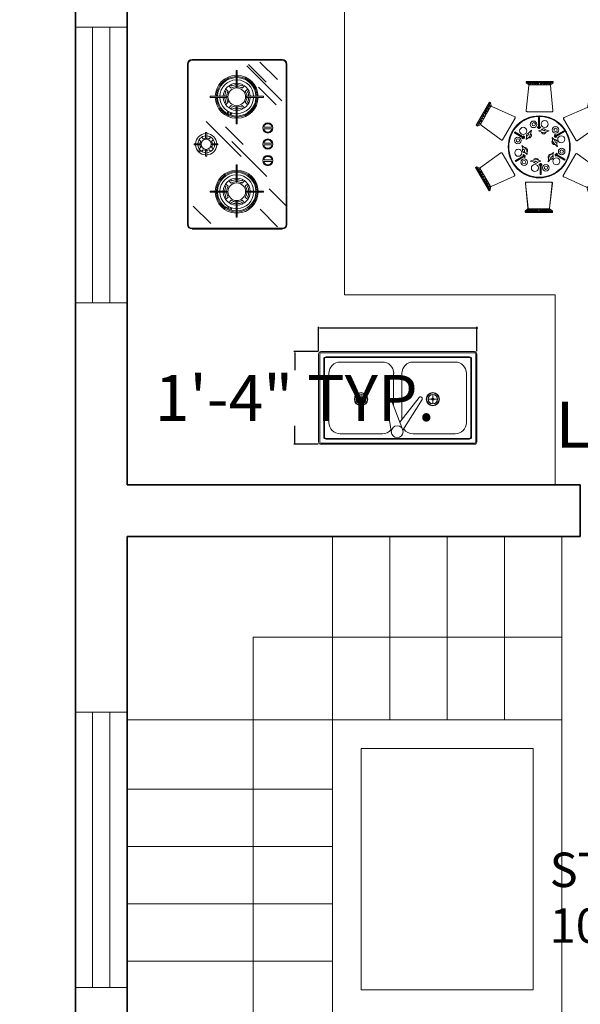
# Model space of a CAD drawing. Units: inches. Extents: x 125 to 976, y 231 to 853.
# Tile 13 of 16: x 557 to 655, y 413 to 584. Entities that reach past the tile are written whole.
import ezdxf

# ---------------------------------------------------------------- set-up
doc = ezdxf.new("R2010")
doc.units = ezdxf.units.IN
doc.header["$MEASUREMENT"] = 0
for name, color, linetype, lineweight in [('A-ANNO-DIMS', 2, 'Continuous', 18), ('A-AREA-IDEN', 7, 'Continuous', 18), ('A-EQPM', 8, 'Continuous', 15), ('A-FLOR-CASE', 32, 'Continuous', 18), ('A-FLOR-FIXT', 9, 'Continuous', 18), ('A-FLOR-STRS', 7, 'Continuous', 18), ('A-GLAZ', 4, 'Continuous', 18), ('A-WALL', 7, 'Continuous', 35), ('Furniture', 8, 'Continuous', 15)]:
    doc.layers.add(name, color=color, linetype=linetype, lineweight=lineweight)
doc.styles.get("Standard").update_dxf_attribs({"font": 'italic8.shx'})
doc.dimstyles.get("Standard").update_dxf_attribs({"dimtxt": 8, "dimasz": 0.18, "dimexe": 0.18, "dimexo": 0.0625, "dimgap": 0.09, "dimtad": 0, "dimtih": 1, "dimtoh": 1, "dimdec": 4, "dimzin": 0, "dimdsep": 46, "dimlunit": 3, "dimtxsty": 'Standard', "dimcen": 0.09, "dimclrt": 4, "dimadec": 0, "dimazin": 0, "dimtfac": 1, "dimtdec": 4, "dimtofl": 0, "dimtmove": 0, "dimatfit": 3, "dimfxl": 1, "dimtolj": 1, "dimtzin": 0, "dimarcsym": 0})

# ---------------------------------------------------------------- blocks, each defined once
blk = doc.blocks.new('DINING-SET-ROUND-6')
for p, q in [((8.8, 22.58), (9.2, 22.26)), ((8.83, 22.8), (8.83, 22.6)), ((13.52, 22.8), (8.83, 22.8)), ((8.83, 22.6), (13.52, 22.6)), ((9.19, 22.53), (9.57, 22.55)), ((9.54, 22.27), (9.19, 22.53)), ((9.57, 22.55), (9.56, 22.32)), ((9.67, 22.56), (9.91, 22.32)), ((9.8, 22.55), (9.89, 22.55)), ((10.04, 22.32), (9.8, 22.55)), ((9.89, 22.55), (10.01, 22.45)), ((9.91, 22.32), (10.04, 22.32)), ((10.01, 22.45), (10.04, 22.48)), ((10.04, 22.48), (10.05, 22.34)), ((10.15, 22.56), (10.39, 22.32)), ((10.28, 22.55), (10.37, 22.55)), ((10.52, 22.32), (10.28, 22.55)), ((10.37, 22.55), (10.49, 22.45)), ((10.39, 22.32), (10.52, 22.32)), ((10.49, 22.45), (10.52, 22.48)), ((10.52, 22.48), (10.54, 22.34)), ((10.63, 22.56), (10.87, 22.32)), ((10.76, 22.55), (10.86, 22.55)), ((11, 22.32), (10.76, 22.55)), ((10.86, 22.55), (10.97, 22.45)), ((10.87, 22.32), (11, 22.32)), ((10.97, 22.45), (11, 22.48)), ((11, 22.48), (11.02, 22.34)), ((11.32, 22.48), (11.31, 22.34)), ((11.32, 22.32), (11.56, 22.55)), ((11.35, 22.45), (11.32, 22.48)), ((11.45, 22.32), (11.32, 22.32)), ((11.47, 22.55), (11.35, 22.45)), ((11.69, 22.56), (11.45, 22.32)), ((11.56, 22.55), (11.47, 22.55)), ((11.8, 22.48), (11.79, 22.34)), ((11.8, 22.32), (12.04, 22.55)), ((11.83, 22.45), (11.8, 22.48)), ((11.93, 22.32), (11.8, 22.32)), ((11.95, 22.55), (11.83, 22.45)), ((12.17, 22.56), (11.93, 22.32)), ((12.04, 22.55), (11.95, 22.55)), ((12.28, 22.48), (12.27, 22.34)), ((12.28, 22.32), (12.52, 22.55)), ((12.32, 22.45), (12.28, 22.48)), ((12.41, 22.32), (12.28, 22.32)), ((12.43, 22.55), (12.32, 22.45)), ((12.65, 22.56), (12.41, 22.32)), ((12.52, 22.55), (12.43, 22.55)), ((12.75, 22.55), (12.77, 22.32)), ((13.13, 22.53), (12.75, 22.55)), ((12.78, 22.27), (13.13, 22.53)), ((13.52, 22.58), (13.12, 22.26)), ((13.52, 22.6), (13.52, 22.8)), ((8.82, 17.72), (9.3, 22.08)), ((9.2, 22.26), (9.54, 22.27)), ((9.46, 22.23), (12.91, 22.23)), ((13.12, 22.26), (12.78, 22.27)), ((13.07, 22.08), (13.49, 17.72)), ((2.44, 19.22), (0.09, 15.16)), ((0.27, 15.05), (2.62, 19.11)), ((2.62, 19.11), (2.44, 19.22)), ((2.63, 19.1), (2.71, 18.6)), ((19.62, 18.97), (19.54, 18.47)), ((19.83, 19.06), (19.65, 18.95)), ((19.65, 18.95), (21.99, 14.9)), ((22.17, 15), (19.83, 19.06)), ((0.91, 15.41), (2.63, 18.4)), ((1.66, 17.16), (1.62, 17.15)), ((1.68, 17.39), (1.63, 17.31)), ((1.63, 17.31), (1.66, 17.16)), ((1.75, 17.07), (1.68, 17.39)), ((1.73, 17.51), (1.82, 17.18)), ((1.82, 17.18), (1.75, 17.07)), ((1.9, 17.58), (1.86, 17.57)), ((1.86, 17.57), (1.97, 17.48)), ((1.92, 17.81), (1.87, 17.73)), ((1.87, 17.73), (1.9, 17.58)), ((1.99, 17.49), (1.92, 17.81)), ((1.97, 17.93), (2.06, 17.6)), ((2.06, 17.6), (1.99, 17.49)), ((2.14, 18), (2.1, 17.99)), ((2.1, 17.99), (2.21, 17.9)), ((2.16, 18.23), (2.11, 18.14)), ((2.11, 18.14), (2.14, 18)), ((2.24, 17.91), (2.16, 18.23)), ((2.21, 18.35), (2.3, 18.02)), ((2.3, 18.02), (2.24, 17.91)), ((2.48, 18.75), (2.27, 18.42)), ((2.27, 18.42), (2.48, 18.32)), ((2.53, 18.31), (2.48, 18.75)), ((2.71, 18.6), (2.53, 18.31)), ((2.84, 18.46), (6.82, 16.65)), ((13.33, 17.54), (8.98, 17.54)), ((15.42, 16.53), (19.43, 18.29)), ((19.54, 18.47), (19.72, 18.18)), ((19.64, 18.23), (21.36, 15.24)), ((19.72, 18.18), (19.77, 18.62)), ((19.77, 18.62), (19.97, 18.29)), ((19.97, 18.29), (19.77, 18.19)), ((20.03, 18.21), (19.95, 17.89)), ((19.95, 17.89), (20.01, 17.77)), ((20.01, 17.77), (20.08, 18.1)), ((20.15, 17.86), (20.03, 17.77)), ((20.08, 18.1), (20.13, 18.01)), ((20.13, 18.01), (20.11, 17.87)), ((20.11, 17.87), (20.15, 17.86)), ((20.28, 17.8), (20.19, 17.47)), ((20.19, 17.47), (20.25, 17.36)), ((20.25, 17.36), (20.33, 17.68)), ((20.39, 17.44), (20.27, 17.35)), ((20.33, 17.68), (20.37, 17.6)), ((20.37, 17.6), (20.35, 17.45)), ((20.35, 17.45), (20.39, 17.44)), ((20.52, 17.38), (20.43, 17.05)), ((20.49, 16.94), (20.57, 17.26)), ((20.57, 17.26), (20.61, 17.18)), ((20.61, 17.18), (20.59, 17.03)), ((0.51, 15.33), (0.69, 15.67)), ((0.91, 15.51), (0.51, 15.33)), ((0.69, 15.67), (0.87, 15.54)), ((0.72, 15.76), (1.05, 15.85)), ((0.75, 15.21), (0.91, 15.51)), ((1.11, 15.96), (0.8, 15.86)), ((0.8, 15.86), (0.85, 15.95)), ((0.85, 15.95), (0.99, 16)), ((0.96, 16.18), (1.29, 16.27)), ((0.97, 16.04), (1.11, 15.98)), ((0.99, 16), (0.97, 16.04)), ((1.35, 16.38), (1.04, 16.28)), ((1.04, 16.28), (1.09, 16.36)), ((1.05, 15.85), (1.11, 15.96)), ((1.09, 16.36), (1.23, 16.41)), ((1.2, 16.59), (1.53, 16.68)), ((1.23, 16.41), (1.21, 16.46)), ((1.21, 16.46), (1.35, 16.4)), ((1.59, 16.79), (1.28, 16.7)), ((1.28, 16.7), (1.33, 16.78)), ((1.29, 16.27), (1.35, 16.38)), ((1.33, 16.78), (1.47, 16.83)), ((1.45, 16.87), (1.59, 16.82)), ((1.47, 16.83), (1.45, 16.87)), ((1.53, 16.68), (1.59, 16.79)), ((1.62, 17.15), (1.73, 17.07)), ((6.9, 16.42), (4.72, 12.66)), ((10.97, 16.52, 0.91), (10.97, 14.61, 0.91)), ((11.03, 16.52, 0.91), (10.97, 16.52, 0.91)), ((11.03, 14.61, 0.91), (11.03, 16.52, 0.91)), ((11.08, 16.52, 0.91), (11.08, 14.61, 0.91)), ((11.14, 16.52, 0.91), (11.08, 16.52, 0.91)), ((11.14, 14.61, 0.91), (11.14, 16.52, 0.91)), ((17.52, 12.54), (15.34, 16.3)), ((20.43, 17.05), (20.49, 16.94)), ((20.63, 17.02), (20.51, 16.94)), ((20.59, 17.03), (20.63, 17.02)), ((20.65, 16.66), (20.97, 16.57)), ((20.72, 16.55), (20.65, 16.66)), ((20.79, 16.74), (20.66, 16.69)), ((21.05, 16.46), (20.72, 16.55)), ((20.78, 16.7), (20.79, 16.74)), ((20.92, 16.65), (20.78, 16.7)), ((20.89, 16.25), (21.21, 16.15)), ((20.96, 16.14), (20.89, 16.25)), ((21.03, 16.33), (20.9, 16.27)), ((20.97, 16.57), (20.92, 16.65)), ((21.29, 16.05), (20.96, 16.14)), ((21.02, 16.28), (21.03, 16.33)), ((21.16, 16.23), (21.02, 16.28)), ((21.13, 15.83), (21.45, 15.73)), ((21.2, 15.72), (21.13, 15.83)), ((21.27, 15.91), (21.14, 15.85)), ((21.21, 16.15), (21.16, 16.23)), ((21.53, 15.63), (21.2, 15.72)), ((21.26, 15.87), (21.27, 15.91)), ((21.4, 15.82), (21.26, 15.87)), ((21.56, 15.54), (21.37, 15.41)), ((21.45, 15.73), (21.4, 15.82)), ((21.74, 15.2), (21.56, 15.54)), ((0.09, 15.16), (0.27, 15.05)), ((0.27, 15.02), (0.75, 15.21)), ((4.49, 12.61), (0.95, 15.2)), ((6.8, 13.9, 0.91), (6.77, 13.85, 0.91)), ((6.77, 13.85, 0.91), (8.43, 12.89, 0.91)), ((8.46, 12.94, 0.91), (6.8, 13.9, 0.91)), ((6.86, 14, 0.91), (6.83, 13.95, 0.91)), ((6.83, 13.95, 0.91), (8.49, 12.99, 0.91)), ((8.52, 13.04, 0.91), (6.86, 14, 0.91)), ((9.74, 14.31, 0.91), (9.23, 13.78, 0.91)), ((9.23, 13.78, 0.91), (9.27, 13.54, 0.91)), ((9.58, 13.56, 0.91), (9.74, 14.31, 0.91)), ((10.81, 14.88, 0.91), (10.81, 14.72, 0.91)), ((10.97, 14.88, 0.91), (10.81, 14.88, 0.91)), ((10.81, 14.72, 0.91), (10.97, 14.72, 0.91)), ((10.97, 14.61, 0.91), (11.03, 14.61, 0.91)), ((11.61, 14.37, 0.91), (10.99, 14.19, 0.91)), ((10.99, 14.19, 0.91), (11.68, 13.89, 0.91)), ((11.08, 14.88, 0.91), (11.03, 14.88, 0.91)), ((11.03, 14.72, 0.91), (11.08, 14.72, 0.91)), ((11.08, 14.61, 0.91), (11.14, 14.61, 0.91)), ((11.31, 14.88, 0.91), (11.14, 14.88, 0.91)), ((11.14, 14.72, 0.91), (11.31, 14.72, 0.91)), ((11.31, 14.72, 0.91), (11.31, 14.88, 0.91)), ((11.94, 14.21, 0.91), (11.61, 14.37, 0.91)), ((11.68, 13.89, 0.91), (12.12, 13.95, 0.91)), ((12.14, 14.36, 0.91), (11.94, 14.21, 0.91)), ((12.12, 13.95, 0.91), (12.85, 14.19, 0.91)), ((12.85, 14.19, 0.91), (12.14, 14.36, 0.91)), ((15.38, 14.23, 0.91), (13.72, 13.27, 0.91)), ((13.75, 13.22, 0.91), (15.41, 14.18, 0.91)), ((15.44, 14.13, 0.91), (13.78, 13.17, 0.91)), ((13.81, 13.12, 0.91), (15.47, 14.08, 0.91)), ((15.41, 14.18, 0.91), (15.38, 14.23, 0.91)), ((15.47, 14.08, 0.91), (15.44, 14.13, 0.91)), ((21.32, 15.03), (17.75, 12.49)), ((21.34, 15.37), (21.74, 15.2)), ((21.5, 15.07), (21.34, 15.37)), ((21.97, 14.89), (21.5, 15.07)), ((21.99, 14.9), (22.17, 15)), ((8.2, 13.02, 0.91), (8.12, 12.89, 0.91)), ((8.12, 12.89, 0.91), (8.26, 12.81, 0.91)), ((8.26, 13.12, 0.91), (8.23, 13.07, 0.91)), ((8.26, 12.81, 0.91), (8.34, 12.95, 0.91)), ((8.37, 13.32, 0.91), (8.29, 13.17, 0.91)), ((8.51, 13.24, 0.91), (8.37, 13.32, 0.91)), ((8.37, 13, 0.91), (8.39, 13.04, 0.91)), ((8.42, 13.1, 0.91), (8.51, 13.24, 0.91)), ((8.43, 12.89, 0.91), (8.46, 12.94, 0.91)), ((8.49, 12.99, 0.91), (8.52, 13.04, 0.91)), ((8.96, 13.32, 0.91), (8.81, 12.7, 0.91)), ((8.81, 12.7, 0.91), (9.41, 13.15, 0.91)), ((9.27, 13.54, 0.91), (8.96, 13.32, 0.91)), ((9.41, 13.15, 0.91), (9.58, 13.56, 0.91)), ((13.84, 12.59, 0.91), (13.37, 13.04, 0.91)), ((13.37, 13.04, 0.91), (13.46, 12.29, 0.91)), ((13.46, 12.29, 0.91), (13.73, 11.94, 0.91)), ((13.72, 13.27, 0.91), (13.75, 13.22, 0.91)), ((13.88, 13.54, 0.91), (13.74, 13.46, 0.91)), ((13.74, 13.46, 0.91), (13.82, 13.33, 0.91)), ((13.78, 13.17, 0.91), (13.81, 13.12, 0.91)), ((13.87, 12.23, 0.91), (13.84, 12.59, 0.91)), ((13.85, 13.27, 0.91), (13.88, 13.23, 0.91)), ((14.09, 12.13, 0.91), (13.87, 12.23, 0.91)), ((13.96, 13.4, 0.91), (13.88, 13.54, 0.91)), ((13.91, 13.18, 0.91), (13.99, 13.03, 0.91)), ((14.01, 13.31, 0.91), (13.99, 13.35, 0.91)), ((13.99, 13.03, 0.91), (14.13, 13.11, 0.91)), ((14.13, 13.11, 0.91), (14.04, 13.25, 0.91)), ((14.3, 11.43, 0.91), (14.09, 12.13, 0.91)), ((0.85, 7.79), (4.42, 10.34)), ((8.08, 11.67, 0.91), (8.28, 10.97, 0.91)), ((8.64, 11.17, 0.91), (8.08, 11.67, 0.91)), ((8.28, 10.97, 0.91), (8.51, 10.88, 0.91)), ((8.51, 10.88, 0.91), (8.54, 10.51, 0.91)), ((8.54, 10.51, 0.91), (9, 10.06, 0.91)), ((8.92, 10.81, 0.91), (8.64, 11.17, 0.91)), ((9, 10.06, 0.91), (8.92, 10.81, 0.91)), ((13.57, 10.41, 0.91), (12.96, 9.95, 0.91)), ((13.41, 9.78, 0.91), (13.57, 10.41, 0.91)), ((13.73, 11.94, 0.91), (14.3, 11.43, 0.91)), ((14.12, 10.3, 0.91), (14.04, 10.16, 0.91)), ((14.25, 10.22, 0.91), (14.12, 10.3, 0.91)), ((4.65, 10.29), (6.83, 6.52)), ((8.57, 9.99, 0.91), (6.91, 9.03, 0.91)), ((6.91, 9.03, 0.91), (6.94, 8.97, 0.91)), ((6.94, 8.97, 0.91), (8.6, 9.93, 0.91)), ((8.62, 9.89, 0.91), (6.96, 8.93, 0.91)), ((6.96, 8.93, 0.91), (6.99, 8.88, 0.91)), ((6.99, 8.88, 0.91), (8.65, 9.84, 0.91)), ((8.38, 10.07, 0.91), (8.25, 10, 0.91)), ((8.25, 10, 0.91), (8.33, 9.85, 0.91)), ((8.36, 9.8, 0.91), (8.39, 9.75, 0.91)), ((8.47, 9.93, 0.91), (8.38, 10.07, 0.91)), ((8.42, 9.7, 0.91), (8.5, 9.57, 0.91)), ((8.53, 9.83, 0.91), (8.5, 9.88, 0.91)), ((8.5, 9.57, 0.91), (8.63, 9.64, 0.91)), ((8.63, 9.64, 0.91), (8.56, 9.78, 0.91)), ((8.6, 9.93, 0.91), (8.57, 9.99, 0.91)), ((8.65, 9.84, 0.91), (8.62, 9.89, 0.91)), ((10.25, 9.16, 0.91), (9.53, 8.92, 0.91)), ((9.53, 8.92, 0.91), (10.24, 8.75, 0.91)), ((10.24, 8.75, 0.91), (10.43, 8.9, 0.91)), ((10.69, 9.22, 0.91), (10.25, 9.16, 0.91)), ((10.43, 8.9, 0.91), (10.77, 8.74, 0.91)), ((11.39, 8.92, 0.91), (10.69, 9.22, 0.91)), ((10.77, 8.74, 0.91), (11.39, 8.92, 0.91)), ((12.79, 9.54, 0.91), (12.64, 8.8, 0.91)), ((12.64, 8.8, 0.91), (13.14, 9.33, 0.91)), ((12.96, 9.95, 0.91), (12.79, 9.54, 0.91)), ((13.11, 9.57, 0.91), (13.41, 9.78, 0.91)), ((13.14, 9.33, 0.91), (13.11, 9.57, 0.91)), ((13.88, 10.12, 0.91), (13.85, 10.07, 0.91)), ((13.85, 10.07, 0.91), (15.52, 9.11, 0.91)), ((13.95, 10.01, 0.91), (13.87, 9.86, 0.91)), ((13.87, 9.86, 0.91), (14, 9.79, 0.91)), ((15.55, 9.16, 0.91), (13.88, 10.12, 0.91)), ((13.94, 10.22, 0.91), (13.91, 10.17, 0.91)), ((13.91, 10.17, 0.91), (15.57, 9.21, 0.91)), ((15.6, 9.26, 0.91), (13.94, 10.22, 0.91)), ((14.01, 10.11, 0.91), (13.98, 10.06, 0.91)), ((14, 9.79, 0.91), (14.09, 9.93, 0.91)), ((14.12, 9.98, 0.91), (14.15, 10.03, 0.91)), ((14.18, 10.08, 0.91), (14.25, 10.22, 0.91)), ((15.28, 6.4), (17.45, 10.17)), ((15.52, 9.11, 0.91), (15.55, 9.16, 0.91)), ((15.57, 9.21, 0.91), (15.6, 9.26, 0.91)), ((17.68, 10.22), (21.22, 7.62)), ((0.18, 7.93), (0, 7.82)), ((0, 7.82), (2.35, 3.77)), ((2.53, 3.87), (0.18, 7.93)), ((0.2, 7.94), (0.68, 7.75)), ((0.43, 7.63), (0.61, 7.29)), ((0.83, 7.45), (0.43, 7.63)), ((0.61, 7.29), (0.8, 7.41)), ((0.64, 7.19), (0.97, 7.11)), ((0.68, 7.75), (0.83, 7.45)), ((0.72, 7.09), (0.77, 7.01)), ((1.04, 6.99), (0.72, 7.09)), ((0.77, 7.01), (0.91, 6.96)), ((2.53, 4.6), (0.81, 7.58)), ((0.9, 6.91), (1.03, 6.97)), ((0.91, 6.96), (0.9, 6.91)), ((0.97, 7.11), (1.04, 6.99)), ((11.23, 8.39, 0.91), (11.07, 8.39, 0.91)), ((11.07, 8.39, 0.91), (11.07, 8.23, 0.91)), ((11.07, 8.23, 0.91), (11.23, 8.23, 0.91)), ((11.29, 8.5, 0.91), (11.23, 8.5, 0.91)), ((11.23, 8.5, 0.91), (11.23, 6.58, 0.91)), ((11.29, 6.58, 0.91), (11.29, 8.5, 0.91)), ((11.35, 8.39, 0.91), (11.29, 8.39, 0.91)), ((11.29, 8.23, 0.91), (11.35, 8.23, 0.91)), ((11.41, 8.5, 0.91), (11.35, 8.5, 0.91)), ((11.35, 8.5, 0.91), (11.35, 6.58, 0.91)), ((11.41, 6.58, 0.91), (11.41, 8.5, 0.91)), ((11.56, 8.39, 0.91), (11.41, 8.39, 0.91)), ((11.41, 8.23, 0.91), (11.56, 8.23, 0.91)), ((11.56, 8.23, 0.91), (11.56, 8.39, 0.91)), ((21.26, 7.41), (19.54, 4.43)), ((21.9, 7.77), (19.55, 3.71)), ((19.73, 3.61), (22.08, 7.67)), ((21.12, 6.98), (21.06, 6.86)), ((21.06, 6.86), (21.37, 6.96)), ((21.45, 7.06), (21.12, 6.98)), ((21.33, 6.88), (21.19, 6.83)), ((21.42, 7.62), (21.27, 7.32)), ((21.27, 7.32), (21.66, 7.5)), ((21.49, 7.15), (21.3, 7.28)), ((21.37, 6.96), (21.33, 6.88)), ((21.9, 7.81), (21.42, 7.62)), ((21.66, 7.5), (21.49, 7.15)), ((22.08, 7.67), (21.9, 7.77)), ((0.88, 6.78), (1.21, 6.69)), ((0.96, 6.67), (1.01, 6.59)), ((1.28, 6.58), (0.96, 6.67)), ((1.01, 6.59), (1.15, 6.54)), ((1.13, 6.36), (1.45, 6.27)), ((1.14, 6.5), (1.27, 6.56)), ((1.15, 6.54), (1.14, 6.5)), ((1.2, 6.26), (1.25, 6.17)), ((1.52, 6.16), (1.2, 6.26)), ((1.21, 6.69), (1.28, 6.58)), ((1.25, 6.17), (1.39, 6.12)), ((1.38, 6.08), (1.51, 6.14)), ((1.39, 6.12), (1.38, 6.08)), ((1.45, 6.27), (1.52, 6.16)), ((1.54, 5.8), (1.66, 5.89)), ((1.58, 5.79), (1.54, 5.8)), ((1.56, 5.65), (1.58, 5.79)), ((1.6, 5.56), (1.56, 5.65)), ((1.68, 5.88), (1.6, 5.56)), ((1.65, 5.44), (1.74, 5.77)), ((1.74, 5.77), (1.68, 5.88)), ((1.78, 5.39), (1.9, 5.47)), ((1.82, 5.37), (1.78, 5.39)), ((1.8, 5.23), (1.82, 5.37)), ((1.85, 5.15), (1.8, 5.23)), ((1.92, 5.47), (1.85, 5.15)), ((1.9, 5.03), (1.98, 5.35)), ((1.98, 5.35), (1.92, 5.47)), ((6.75, 6.3), (2.74, 4.53)), ((8.84, 5.28), (13.19, 5.28)), ((8.89, 5.26), (13.23, 5.26)), ((11.23, 6.58, 0.91), (11.29, 6.58, 0.91)), ((11.35, 6.58, 0.91), (11.41, 6.58, 0.91)), ((19.33, 4.36), (15.35, 6.18)), ((20.11, 5.22), (20.18, 5.34)), ((20.2, 4.9), (20.11, 5.22)), ((20.18, 5.34), (20.25, 5.01)), ((20.31, 5.26), (20.2, 5.34)), ((20.27, 5.24), (20.31, 5.26)), ((20.3, 5.1), (20.27, 5.24)), ((20.35, 5.64), (20.42, 5.75)), ((20.44, 5.31), (20.35, 5.64)), ((20.42, 5.75), (20.49, 5.43)), ((20.56, 5.67), (20.44, 5.76)), ((20.49, 5.43), (20.54, 5.51)), ((20.51, 5.66), (20.56, 5.67)), ((20.54, 5.51), (20.51, 5.66)), ((20.64, 6.14), (20.58, 6.03)), ((20.58, 6.03), (20.89, 6.13)), ((20.72, 5.95), (20.58, 6.01)), ((20.97, 6.23), (20.64, 6.14)), ((20.84, 6.04), (20.7, 5.99)), ((20.7, 5.99), (20.72, 5.95)), ((20.88, 6.56), (20.82, 6.45)), ((20.82, 6.45), (21.13, 6.54)), ((20.96, 6.37), (20.82, 6.43)), ((20.89, 6.13), (20.84, 6.04)), ((21.21, 6.65), (20.88, 6.56)), ((21.08, 6.46), (20.94, 6.41)), ((20.94, 6.41), (20.96, 6.37)), ((21.2, 6.78), (21.06, 6.84)), ((21.13, 6.54), (21.08, 6.46)), ((21.19, 6.83), (21.2, 6.78)), ((2.02, 4.97), (2.14, 5.06)), ((2.07, 4.96), (2.02, 4.97)), ((2.04, 4.81), (2.07, 4.96)), ((2.09, 4.73), (2.04, 4.81)), ((2.16, 5.05), (2.09, 4.73)), ((2.14, 4.61), (2.22, 4.94)), ((2.22, 4.94), (2.16, 5.05)), ((2.2, 4.53), (2.4, 4.63)), ((2.4, 4.21), (2.2, 4.53)), ((2.35, 3.77), (2.53, 3.87)), ((2.45, 4.64), (2.4, 4.21)), ((2.63, 4.36), (2.45, 4.64)), ((2.56, 3.85), (2.63, 4.36)), ((9.1, 0.74), (8.68, 5.1)), ((9.14, 0.73), (8.73, 5.09)), ((13.35, 5.1), (12.87, 0.74)), ((13.39, 5.09), (12.91, 0.72)), ((19.46, 4.23), (19.64, 4.51)), ((19.54, 3.72), (19.46, 4.23)), ((19.55, 3.71), (19.73, 3.61)), ((19.64, 4.51), (19.69, 4.08)), ((19.9, 4.4), (19.69, 4.5)), ((19.69, 4.08), (19.9, 4.4)), ((19.87, 4.81), (19.94, 4.92)), ((19.96, 4.48), (19.87, 4.81)), ((19.94, 4.92), (20.01, 4.6)), ((20.07, 4.84), (19.96, 4.92)), ((20.01, 4.6), (20.06, 4.68)), ((20.03, 4.83), (20.07, 4.84)), ((20.06, 4.68), (20.03, 4.83)), ((20.25, 5.01), (20.3, 5.1)), ((8.65, 0.24), (9.05, 0.57)), ((8.65, 0.23), (8.65, 0.02)), ((13.34, 0.23), (8.65, 0.23)), ((8.65, 0.02), (13.34, 0.02)), ((8.69, 0.23), (9.09, 0.55)), ((8.69, 0.21), (8.69, 0)), ((13.38, 0.21), (8.69, 0.21)), ((8.69, 0), (13.38, 0)), ((9.39, 0.55), (9.04, 0.29)), ((9.04, 0.29), (9.42, 0.28)), ((9.05, 0.57), (9.39, 0.55)), ((9.43, 0.53), (9.08, 0.28)), ((9.08, 0.28), (9.46, 0.26)), ((9.09, 0.55), (9.43, 0.53)), ((12.71, 0.6), (9.26, 0.6)), ((12.75, 0.58), (9.3, 0.58)), ((9.42, 0.28), (9.41, 0.5)), ((9.46, 0.26), (9.45, 0.49)), ((9.52, 0.26), (9.76, 0.5)), ((9.56, 0.25), (9.8, 0.49)), ((9.89, 0.5), (9.65, 0.28)), ((9.65, 0.28), (9.74, 0.28)), ((9.93, 0.49), (9.69, 0.26)), ((9.69, 0.26), (9.78, 0.26)), ((9.74, 0.28), (9.85, 0.37)), ((9.76, 0.5), (9.89, 0.5)), ((9.78, 0.26), (9.9, 0.36)), ((9.8, 0.49), (9.93, 0.49)), ((9.85, 0.37), (9.89, 0.34)), ((9.89, 0.34), (9.9, 0.49)), ((9.9, 0.36), (9.93, 0.33)), ((9.93, 0.33), (9.94, 0.47)), ((10, 0.26), (10.24, 0.5)), ((10.04, 0.25), (10.28, 0.49)), ((10.37, 0.5), (10.13, 0.28)), ((10.13, 0.28), (10.22, 0.28)), ((10.41, 0.49), (10.17, 0.26)), ((10.17, 0.26), (10.27, 0.26)), ((10.22, 0.28), (10.34, 0.37)), ((10.24, 0.5), (10.37, 0.5)), ((10.27, 0.26), (10.38, 0.36)), ((10.28, 0.49), (10.41, 0.49)), ((10.34, 0.37), (10.37, 0.34)), ((10.37, 0.34), (10.38, 0.49)), ((10.38, 0.36), (10.41, 0.33)), ((10.41, 0.33), (10.43, 0.47)), ((10.48, 0.26), (10.72, 0.5)), ((10.52, 0.25), (10.76, 0.49)), ((10.85, 0.5), (10.61, 0.28)), ((10.61, 0.28), (10.71, 0.28)), ((10.89, 0.49), (10.65, 0.26)), ((10.65, 0.26), (10.75, 0.26)), ((10.71, 0.28), (10.82, 0.37)), ((10.72, 0.5), (10.85, 0.5)), ((10.75, 0.26), (10.86, 0.36)), ((10.76, 0.49), (10.89, 0.49)), ((10.82, 0.37), (10.85, 0.34)), ((10.85, 0.34), (10.87, 0.49)), ((10.86, 0.36), (10.89, 0.33)), ((10.89, 0.33), (10.91, 0.47)), ((11.17, 0.34), (11.15, 0.49)), ((11.17, 0.5), (11.41, 0.28)), ((11.3, 0.5), (11.17, 0.5)), ((11.2, 0.37), (11.17, 0.34)), ((11.21, 0.33), (11.2, 0.47)), ((11.31, 0.28), (11.2, 0.37)), ((11.21, 0.49), (11.45, 0.26)), ((11.34, 0.49), (11.21, 0.49)), ((11.24, 0.36), (11.21, 0.33)), ((11.36, 0.26), (11.24, 0.36)), ((11.54, 0.26), (11.3, 0.5)), ((11.41, 0.28), (11.31, 0.28)), ((11.58, 0.25), (11.34, 0.49)), ((11.45, 0.26), (11.36, 0.26)), ((11.65, 0.34), (11.64, 0.49)), ((11.65, 0.5), (11.89, 0.28)), ((11.78, 0.5), (11.65, 0.5)), ((11.68, 0.37), (11.65, 0.34)), ((11.69, 0.33), (11.68, 0.47)), ((11.8, 0.28), (11.68, 0.37)), ((11.69, 0.49), (11.93, 0.26)), ((11.82, 0.49), (11.69, 0.49)), ((11.73, 0.36), (11.69, 0.33)), ((11.84, 0.26), (11.73, 0.36)), ((12.02, 0.26), (11.78, 0.5)), ((11.89, 0.28), (11.8, 0.28)), ((12.06, 0.25), (11.82, 0.49)), ((11.93, 0.26), (11.84, 0.26)), ((12.13, 0.34), (12.12, 0.49)), ((12.13, 0.5), (12.37, 0.28)), ((12.26, 0.5), (12.13, 0.5)), ((12.17, 0.37), (12.13, 0.34)), ((12.17, 0.33), (12.16, 0.47)), ((12.17, 0.49), (12.42, 0.26)), ((12.3, 0.49), (12.17, 0.49)), ((12.28, 0.28), (12.17, 0.37)), ((12.21, 0.36), (12.17, 0.33)), ((12.32, 0.26), (12.21, 0.36)), ((12.5, 0.26), (12.26, 0.5)), ((12.37, 0.28), (12.28, 0.28)), ((12.54, 0.25), (12.3, 0.49)), ((12.42, 0.26), (12.32, 0.26)), ((12.6, 0.28), (12.61, 0.5)), ((12.98, 0.29), (12.6, 0.28)), ((12.97, 0.57), (12.63, 0.55)), ((12.63, 0.55), (12.98, 0.29)), ((12.64, 0.26), (12.66, 0.49)), ((13.02, 0.28), (12.64, 0.26)), ((13.01, 0.55), (12.67, 0.53)), ((12.67, 0.53), (13.02, 0.28)), ((13.37, 0.24), (12.97, 0.57)), ((13.41, 0.23), (13.01, 0.55)), ((13.34, 0.02), (13.34, 0.23)), ((13.38, 0), (13.38, 0.21))]:
    blk.add_line(p, q)
for centre, radius in [((11.09, 11.41), 5.4), ((11.09, 11.41), 5.3), ((10.11, 15.33, 0.91), 0.572), ((10.13, 15.34, 0.91), 0.295), ((12.04, 15.38, 0.91), 0.616), ((8.3, 14.2, 0.91), 0.616), ((13.92, 14.37, 0.91), 0.572), ((13.94, 14.37, 0.91), 0.295), ((7.38, 12.51, 0.91), 0.572), ((7.38, 12.53, 0.91), 0.295), ((14.93, 12.73, 0.91), 0.616), ((7.45, 10.38, 0.91), 0.616), ((15, 10.59, 0.91), 0.572), ((15, 10.58, 0.91), 0.295), ((8.45, 8.73, 0.91), 0.572), ((8.44, 8.74, 0.91), 0.295), ((14.08, 8.9, 0.91), 0.616), ((10.34, 7.73, 0.91), 0.616), ((12.26, 7.77, 0.91), 0.572), ((12.25, 7.77, 0.91), 0.295)]:
    blk.add_circle(centre, radius)
for centre, radius, start, end in [((9.46, 22.07), 0.16, 90, 173.7428), ((12.91, 22.07), 0.16, 5.4801, 90), ((2.77, 18.32), 0.16, 65.4801, 150), ((8.98, 17.7), 0.16, 173.7428, 270), ((13.33, 17.7), 0.16, 270, 5.4801), ((19.5, 18.15), 0.16, 30, 113.7428), ((6.76, 16.5), 0.16, 330, 65.4801), ((15.48, 16.38), 0.16, 113.7428, 210), ((1.05, 15.33), 0.16, 150, 233.7428), ((9.3, 13.42, 0.91), 0.448, 86.6641, 214.1442), ((9.3, 13.42, 0.91), 0.448, 257.0611, 44.0662), ((11.86, 14.13, 0.91), 0.448, 197.0611, 344.0662), ((11.86, 14.13, 0.91), 0.448, 26.6641, 154.1442), ((21.22, 15.16), 0.16, 305.4801, 30), ((4.58, 12.74), 0.16, 233.7428, 330), ((13.76, 12.26, 0.91), 0.448, 137.0611, 284.0662), ((13.76, 12.26, 0.91), 0.448, 326.6641, 94.1442), ((17.66, 12.62), 0.16, 210, 305.4801), ((4.52, 10.21), 0.16, 30, 125.4801), ((8.62, 10.85, 0.91), 0.448, 146.6641, 274.1442), ((8.62, 10.85, 0.91), 0.448, 317.0611, 104.0662), ((10.51, 8.98, 0.91), 0.448, 17.0611, 164.0662), ((10.51, 8.98, 0.91), 0.448, 206.6641, 334.1442), ((13.08, 9.68, 0.91), 0.448, 77.0611, 224.0662), ((13.08, 9.68, 0.91), 0.448, 266.6641, 34.1442), ((17.59, 10.09), 0.16, 53.7428, 150), ((0.95, 7.66), 0.16, 125.4801, 210), ((21.13, 7.49), 0.16, 330, 53.7428), ((6.69, 6.44), 0.16, 293.7428, 30), ((8.84, 5.12), 0.16, 90, 185.4801), ((8.89, 5.1), 0.16, 90, 185.4801), ((13.19, 5.12), 0.16, 353.7428, 90), ((13.23, 5.1), 0.16, 353.7428, 90), ((15.41, 6.32), 0.16, 150, 245.4801), ((2.67, 4.68), 0.16, 210, 293.7428), ((19.4, 4.51), 0.16, 245.4801, 330), ((9.26, 0.76), 0.16, 185.4801, 270), ((9.3, 0.74), 0.16, 185.4801, 270), ((12.71, 0.76), 0.16, 270, 353.7428), ((12.75, 0.74), 0.16, 270, 353.7428)]:
    blk.add_arc(centre, radius, start, end)
blk = doc.blocks.new('SINK-DOUBLE')
for p, q in [((0, 15.74), (0, 0.39)), ((0.2, 15.74), (0.2, 0.39)), ((27.17, 16.14), (0.4, 16.14)), ((27.17, 15.94), (0.4, 15.94)), ((27.37, 0.39), (27.37, 15.74)), ((27.56, 0.39), (27.56, 15.74)), ((0.91, 14.84), (0.91, 1.3)), ((1.03, 14.84), (1.03, 1.3)), ((26.26, 15.23), (1.3, 15.23)), ((26.26, 15.11), (1.3, 15.11)), ((11.11, 14.33), (3.78, 14.33)), ((23.78, 14.33), (16.46, 14.33)), ((26.54, 1.3), (26.54, 14.84)), ((26.66, 1.3), (26.66, 14.84)), ((1.81, 12.36), (1.81, 3.78)), ((13.07, 6.7), (13.07, 12.36)), ((14.49, 12.36), (14.49, 4.26)), ((25.75, 3.78), (25.75, 12.36)), ((7.39, 8.06), (7.39, 8.65)), ((19.9, 8.06), (19.9, 8.65)), ((7.18, 7.86), (6.59, 7.86)), ((7.39, 7.65), (7.39, 7.06)), ((7.59, 7.86), (8.18, 7.86)), ((11.9, 7.12), (12.69, 1.93)), ((12.59, 7.48), (12.04, 7.34)), ((14.68, 2.43), (12.83, 7.36)), ((14.16, 3.83), (17.49, 8.16)), ((14.68, 2.43), (18.03, 7.78)), ((17.92, 8.22), (17.95, 8.2)), ((19.7, 7.86), (19.11, 7.86)), ((19.9, 7.65), (19.9, 7.06)), ((20.11, 7.86), (20.7, 7.86)), ((3.78, 1.81), (11.11, 1.81)), ((16.46, 1.81), (23.78, 1.81)), ((0.4, 0.19), (27.17, 0.19)), ((1.3, 1.02), (26.26, 1.02)), ((1.3, 0.9), (26.26, 0.9)), ((0.4, 0), (27.17, 0))]:
    blk.add_line(p, q)
for centre, radius in [((7.39, 7.86), 1.16), ((7.39, 7.86), 1.1), ((7.39, 7.86), 0.83), ((7.39, 7.86), 0.794), ((19.9, 7.86), 1.16), ((19.9, 7.86), 1.1), ((19.9, 7.86), 0.83), ((19.9, 7.86), 0.794), ((7.39, 7.86), 0.204), ((7.39, 7.86), 0.0958), ((19.9, 7.86), 0.204), ((19.9, 7.86), 0.0958), ((13.69, 2.18), 1.03)]:
    blk.add_circle(centre, radius)
for centre, radius, start, end in [((0.4, 15.74), 0.394, 90, 180), ((0.4, 15.74), 0.197, 90, 180), ((27.17, 15.74), 0.394, 0, 90), ((27.17, 15.74), 0.197, 0, 90), ((1.3, 14.84), 0.394, 90, 180), ((1.3, 14.84), 0.276, 90, 180), ((3.78, 12.36), 1.97, 90, 180), ((11.11, 12.36), 1.97, 0, 90), ((16.46, 12.36), 1.97, 90, 180), ((23.78, 12.36), 1.97, 0, 90), ((26.26, 14.84), 0.394, 0, 90), ((26.26, 14.84), 0.276, 0, 90), ((12.09, 7.15), 0.197, 104.3233, 188.6985), ((12.64, 7.29), 0.197, 20.6498, 104.3233), ((17.74, 7.97), 0.315, 53.6309, 142.4185), ((17.76, 7.95), 0.315, 327.9301, 53.6309), ((3.78, 3.78), 1.97, 180, 270), ((23.78, 3.78), 1.97, 270, 0), ((11.11, 3.78), 1.97, 270, 319.575), ((16.46, 3.78), 1.97, 214.0864, 270), ((0.4, 0.39), 0.394, 180, 270), ((0.4, 0.39), 0.197, 180, 270), ((1.3, 1.3), 0.394, 180, 270), ((1.3, 1.3), 0.276, 180, 270), ((26.26, 1.3), 0.276, 270, 0), ((26.26, 1.3), 0.394, 270, 0), ((27.17, 0.39), 0.197, 270, 0), ((27.17, 0.39), 0.394, 270, 0)]:
    blk.add_arc(centre, radius, start, end)
blk = doc.blocks.new('COOKTOP-3BURNER')
for p, q in [((16.54, 29.53), (0.79, 29.53)), ((16.54, 29.41), (0.79, 29.41)), ((0, 28.74), (0, 0.79)), ((0.12, 28.74), (0.12, 0.79)), ((8.48, 24.8), (8.48, 27.63)), ((8.48, 27.63), (8.68, 27.63)), ((8.68, 24.8), (8.68, 27.63)), ((16.45, 22.35), (10.36, 28.44)), ((13.7, 25.61), (10.65, 28.66)), ((15.67, 26.04), (12.63, 29.08)), ((17.21, 0.79), (17.21, 28.74)), ((17.33, 0.79), (17.33, 28.74)), ((6.48, 24.12), (6.69, 23.92)), ((6.65, 24.4), (7.08, 23.97)), ((7.21, 24.95), (7.63, 24.53)), ((7.49, 25.12), (7.69, 24.92)), ((9.67, 25.12), (9.46, 24.92)), ((9.95, 24.95), (9.52, 24.53)), ((10.5, 24.4), (10.08, 23.97)), ((10.67, 24.12), (10.47, 23.92)), ((15.44, 21.65), (12.39, 24.7)), ((6.81, 23.13), (3.94, 23.13)), ((3.94, 23.13), (3.94, 22.93)), ((6.81, 22.93), (3.94, 22.93)), ((10.35, 23.13), (13.24, 23.13)), ((10.35, 22.93), (13.24, 22.93)), ((13.24, 23.13), (13.24, 22.93)), ((6.69, 22.14), (6.48, 21.94)), ((7.08, 22.09), (6.65, 21.66)), ((7.63, 21.53), (7.21, 21.1)), ((7.69, 21.14), (7.49, 20.93)), ((8.48, 21.26), (8.48, 18.35)), ((8.68, 21.26), (8.68, 18.35)), ((9.46, 21.14), (9.67, 20.93)), ((9.52, 21.53), (9.95, 21.1)), ((10.08, 22.09), (10.5, 21.66)), ((10.47, 22.14), (10.67, 21.94)), ((9.35, 12.64), (3.25, 18.73)), ((9.7, 14.73), (6.65, 17.78)), ((8.48, 18.35), (8.68, 18.35)), ((13.4, 17.77), (14.61, 17.77)), ((13.4, 17.46), (14.61, 17.46)), ((2.31, 15.27), (2.02, 15.56)), ((2.75, 15.72), (2.47, 16)), ((3.16, 16.82), (3.36, 16.82)), ((3.16, 15.84), (3.16, 16.82)), ((3.36, 15.84), (3.36, 16.82)), ((4.05, 16), (3.76, 15.72)), ((4.5, 15.56), (4.21, 15.27)), ((1.16, 14.86), (1.16, 14.67)), ((2.18, 14.86), (1.16, 14.86)), ((2.18, 14.67), (1.16, 14.67)), ((2.31, 14.26), (2.02, 13.97)), ((2.75, 13.81), (2.47, 13.53)), ((4.05, 13.53), (3.76, 13.81)), ((4.5, 13.97), (4.21, 14.26)), ((4.34, 14.86), (5.29, 14.86)), ((4.34, 14.67), (5.29, 14.67)), ((5.29, 14.86), (5.29, 14.67)), ((13.81, 9.14), (7.72, 15.23)), ((13.4, 14.96), (14.61, 14.96)), ((13.4, 14.65), (14.61, 14.65)), ((3.16, 13.69), (3.16, 12.69)), ((3.36, 12.69), (3.16, 12.69)), ((3.36, 13.69), (3.36, 12.69)), ((13.4, 12.07), (14.61, 12.07)), ((8.48, 11.18), (8.68, 11.18)), ((8.48, 8.27), (8.48, 11.18)), ((8.68, 8.27), (8.68, 11.18)), ((13.4, 11.76), (14.61, 11.76)), ((7.69, 8.39), (7.49, 8.59)), ((9.46, 8.39), (9.67, 8.59)), ((6.69, 7.39), (6.48, 7.59)), ((7.08, 7.44), (6.65, 7.87)), ((7.63, 8), (7.21, 8.42)), ((9.52, 8), (9.95, 8.42)), ((10.08, 7.44), (10.5, 7.87)), ((10.47, 7.39), (10.67, 7.59)), ((17.27, 3.97), (14.22, 7.02)), ((6.81, 6.6), (3.94, 6.6)), ((3.94, 6.4), (3.94, 6.6)), ((6.81, 6.4), (3.94, 6.4)), ((6.48, 5.41), (6.69, 5.61)), ((6.65, 5.13), (7.08, 5.56)), ((10.5, 5.13), (10.08, 5.56)), ((10.35, 6.6), (13.24, 6.6)), ((10.35, 6.4), (13.24, 6.4)), ((10.67, 5.41), (10.47, 5.61)), ((13.24, 6.4), (13.24, 6.6)), ((4.07, 0.94), (1.02, 3.99)), ((7.21, 4.57), (7.63, 5)), ((7.49, 4.4), (7.69, 4.61)), ((8.48, 4.93), (8.48, 2.09)), ((8.68, 4.93), (8.68, 2.09)), ((9.67, 4.4), (9.46, 4.61)), ((9.95, 4.57), (9.52, 5)), ((15.71, 0.4), (12.67, 3.44)), ((8.48, 2.09), (8.68, 2.09)), ((0.79, 0.12), (16.54, 0.12)), ((0.79, 0), (16.54, 0))]:
    blk.add_line(p, q)
for centre, radius in [((8.58, 23.03), 1.54), ((7.06, 20.26), 0.147), ((7.58, 20.04), 0.147), ((14, 17.61), 0.886), ((14, 17.61), 0.846), ((3.26, 14.76), 0.881), ((14, 14.8), 0.886), ((14, 14.8), 0.846), ((2.12, 13.62), 0.147), ((14, 11.92), 0.886), ((14, 11.92), 0.846), ((8.58, 6.5), 1.54), ((7.03, 3.73), 0.147), ((7.55, 3.51), 0.147)]:
    blk.add_circle(centre, radius)
for centre, radius, start, end in [((0.79, 28.74), 0.787, 90, 180), ((0.79, 28.74), 0.669, 90, 180), ((16.54, 28.74), 0.787, 0, 90), ((16.54, 28.74), 0.669, 0, 90), ((8.58, 23.03), 3.74, 91.5918, 178.4082), ((8.58, 23.03), 3.54, 91.5918, 178.4082), ((8.58, 23.03), 3.35, 91.6854, 178.3146), ((8.58, 23.03), 2.95, 91.9102, 178.0898), ((8.58, 23.03), 3.74, 1.5918, 88.4082), ((8.58, 23.03), 3.54, 1.5918, 88.4082), ((8.58, 23.03), 3.35, 1.6854, 88.3146), ((8.58, 23.03), 2.95, 1.9102, 88.0898), ((8.58, 23.03), 2.36, 92.388, 177.612), ((8.58, 23.03), 1.77, 93.1847, 122.1604), ((8.58, 23.03), 2.09, 92.7036, 115.1461), ((8.58, 24.82), 0.102, 194.2945, 345.7055), ((8.58, 23.03), 2.36, 2.388, 87.612), ((8.58, 23.03), 2.09, 64.8539, 87.2964), ((8.58, 23.03), 1.77, 57.8396, 86.8153), ((8.58, 23.03), 3.74, 181.5918, 268.4082), ((8.58, 23.03), 3.54, 181.5918, 268.4082), ((8.58, 23.03), 3.35, 181.6854, 268.3146), ((8.58, 23.03), 2.95, 181.9102, 268.0898), ((8.58, 23.03), 2.36, 182.388, 267.612), ((8.58, 23.03), 2.09, 154.8539, 177.2964), ((8.58, 23.03), 2.09, 182.7036, 205.1461), ((8.58, 23.03), 1.77, 147.8396, 176.8153), ((6.8, 23.03), 0.0987, 273.9579, 86.0421), ((8.58, 23.03), 1.77, 183.1847, 212.1604), ((8.58, 23.03), 2.36, 272.388, 357.612), ((8.58, 23.03), 3.54, 271.5918, 358.4082), ((8.58, 23.03), 3.35, 271.6854, 358.3146), ((8.58, 23.03), 2.95, 271.9102, 358.0898), ((8.58, 23.03), 3.74, 271.5918, 358.4082), ((8.58, 23.03), 1.77, 3.1847, 32.1604), ((8.58, 23.03), 1.77, 327.8396, 356.8153), ((10.38, 23.03), 0.103, 107.9418, 252.0582), ((8.58, 23.03), 2.09, 2.7036, 25.1461), ((8.58, 23.03), 2.09, 334.8539, 357.2964), ((8.58, 23.03), 1.77, 237.8396, 266.8153), ((8.58, 23.03), 2.09, 244.8539, 267.2964), ((8.58, 21.23), 0.104, 18.412, 161.588), ((8.58, 23.03), 1.77, 273.1847, 302.1604), ((8.58, 23.03), 2.09, 272.7036, 295.1461), ((14, 17.61), 0.728, 21.3237, 158.6763), ((13.4, 17.85), 0.0787, 158.6763, 270), ((13.4, 17.38), 0.0787, 90, 201.3237), ((14, 17.61), 0.728, 201.3237, 338.6763), ((14.61, 17.85), 0.0787, 270, 21.3237), ((14.61, 17.38), 0.0787, 338.6763, 90), ((3.26, 14.76), 1.86, 93.0255, 176.9745), ((3.26, 14.76), 1.47, 93.8363, 176.1637), ((3.26, 14.76), 1.08, 95.206, 118.0021), ((3.26, 15.85), 0.0992, 187.2236, 352.7764), ((3.26, 14.76), 1.86, 3.0255, 86.9745), ((3.26, 14.76), 1.47, 3.8363, 86.1637), ((3.26, 14.76), 1.08, 61.9979, 84.794), ((14, 14.8), 0.728, 21.3237, 158.6763), ((3.26, 14.76), 1.86, 183.0255, 266.9745), ((3.26, 14.76), 1.47, 183.8363, 266.1637), ((2.17, 14.76), 0.0994, 277.9505, 82.0495), ((3.26, 14.76), 1.08, 151.9979, 174.797), ((3.26, 14.76), 1.08, 185.203, 208.0021), ((3.26, 14.76), 1.08, 241.9979, 264.8384), ((3.26, 13.66), 0.103, 17.6318, 162.3682), ((3.26, 14.76), 1.86, 273.0255, 356.9745), ((3.26, 14.76), 1.47, 273.8363, 356.1637), ((3.26, 14.76), 1.08, 275.1616, 298.0021), ((3.26, 14.76), 1.08, 5.2431, 28.0021), ((3.26, 14.76), 1.08, 331.9979, 354.7569), ((4.33, 14.76), 0.0985, 88.3317, 271.6683), ((13.4, 15.04), 0.0787, 158.6763, 270), ((13.4, 14.57), 0.0787, 90, 201.3237), ((14, 14.8), 0.728, 201.3237, 338.6763), ((14.61, 15.04), 0.0787, 270, 21.3237), ((14.61, 14.57), 0.0787, 338.6763, 90), ((14, 11.92), 0.728, 21.3237, 158.6763), ((13.4, 12.15), 0.0787, 158.6763, 270), ((14.61, 12.15), 0.0787, 270, 21.3237), ((13.4, 11.68), 0.0787, 90, 201.3237), ((14, 11.92), 0.728, 201.3237, 338.6763), ((14.61, 11.68), 0.0787, 338.6763, 90), ((8.58, 6.5), 3.74, 91.5918, 178.4082), ((8.58, 6.5), 3.54, 91.5918, 178.4082), ((8.58, 6.5), 3.35, 91.6854, 178.3146), ((8.58, 6.5), 2.95, 91.9102, 178.0898), ((8.58, 6.5), 2.36, 92.388, 177.612), ((8.58, 6.5), 2.09, 92.7036, 115.1461), ((8.58, 6.5), 3.74, 1.5918, 88.4082), ((8.58, 6.5), 3.54, 1.5918, 88.4082), ((8.58, 6.5), 3.35, 1.6854, 88.3146), ((8.58, 6.5), 2.95, 1.9102, 88.0898), ((8.58, 6.5), 2.36, 2.388, 87.612), ((8.58, 6.5), 2.09, 64.8539, 87.2964), ((8.58, 6.5), 2.09, 154.8539, 177.2964), ((8.58, 6.5), 1.77, 147.8396, 176.8153), ((8.58, 6.5), 1.77, 93.1847, 122.1604), ((8.58, 8.31), 0.105, 200.5507, 339.4493), ((8.58, 6.5), 1.77, 57.8396, 86.8153), ((8.58, 6.5), 1.77, 3.1847, 32.1604), ((8.58, 6.5), 2.09, 2.7036, 25.1461), ((8.58, 6.5), 3.74, 181.5918, 268.4082), ((8.58, 6.5), 3.54, 181.5918, 268.4082), ((8.58, 6.5), 3.35, 181.6854, 268.3146), ((8.58, 6.5), 2.95, 181.9102, 268.0898), ((8.58, 6.5), 2.36, 182.388, 267.612), ((8.58, 6.5), 2.09, 182.7036, 205.1461), ((6.8, 6.5), 0.0991, 276.7354, 83.2646), ((8.58, 6.5), 1.77, 183.1847, 212.1604), ((8.58, 6.5), 2.95, 271.9102, 358.0898), ((8.58, 6.5), 2.36, 272.388, 357.612), ((8.58, 6.5), 3.35, 271.6854, 358.3146), ((8.58, 6.5), 3.54, 271.5918, 358.4082), ((8.58, 6.5), 3.74, 271.5918, 358.4082), ((8.58, 6.5), 1.77, 327.8396, 356.8153), ((10.39, 6.5), 0.106, 111.7885, 248.2115), ((8.58, 6.5), 2.09, 334.8539, 357.2964), ((8.58, 6.5), 1.77, 237.8396, 266.8153), ((8.58, 6.5), 2.09, 244.8539, 267.2964), ((8.58, 4.7), 0.104, 18.751, 161.249), ((8.58, 6.5), 1.77, 273.1847, 302.1604), ((8.58, 6.5), 2.09, 272.7036, 295.1461), ((0.79, 0.79), 0.787, 180, 270), ((0.79, 0.79), 0.669, 180, 270), ((16.54, 0.79), 0.669, 270, 0), ((16.54, 0.79), 0.787, 270, 0)]:
    blk.add_arc(centre, radius, start, end)
blk = doc.blocks.new('WINDOW-48IN')
for p, q in [((0, 0), (0, 48)), ((0, 48), (9, 48)), ((3, 0), (3, 48)), ((6, 0), (6, 48)), ((9, 48), (9, 0)), ((9, 0), (0, 0))]:
    blk.add_line(p, q)
blk = doc.blocks.new('*D38')
at = {"layer": 'A-ANNO-DIMS', "color": 0, "lineweight": -2, "transparency": 16777216}
for p, q in [((694.22, 533.1), (700.18, 533.1)), ((700, 532.92), (700, 518.46)), ((700, 494.28), (700, 508.75)), ((694.22, 494.1), (700.18, 494.1))]:
    blk.add_line(p, q, dxfattribs=at)
at = {"layer": 'A-ANNO-DIMS', "color": 0, "transparency": 16777216}
for points in [[(699.97, 532.92), (700.03, 532.92), (700, 533.1)], [(699.97, 494.28), (700.03, 494.28), (700, 494.1)]]:
    blk.add_solid(points, dxfattribs=at)
at = {"layer": 'Defpoints', "color": 0, "transparency": 16777216}
for p in [(694.15, 533.1), (700, 533.1), (694.15, 494.1)]:
    blk.add_point(p, dxfattribs=at)
at = {"layer": 'A-ANNO-DIMS', "color": 4, "transparency": 16777216, "insert": (700, 513.6), "char_height": 8, "attachment_point": 5}
blk.add_mtext('\\A1;LH DOOR 3\'-3" TYP.', dxfattribs=at)
blk = doc.blocks.new('*D48')
at = {"layer": 'A-ANNO-DIMS', "color": 0, "lineweight": -2, "transparency": 16777216}
for p, q in [((609.57, 526.38), (609.57, 530.63)), ((609.75, 530.45), (636.95, 530.45)), ((637.13, 526.38), (637.13, 530.63)), ((637.13, 530.45), (637.31, 530.45))]:
    blk.add_line(p, q, dxfattribs=at)
at = {"layer": 'A-ANNO-DIMS', "color": 0, "transparency": 16777216}
for points in [[(609.75, 530.48), (609.75, 530.42), (609.57, 530.45)], [(636.95, 530.48), (636.95, 530.42), (637.13, 530.45)]]:
    blk.add_solid(points, dxfattribs=at)
at = {"layer": 'Defpoints', "color": 0, "transparency": 16777216}
for p in [(637.13, 530.45), (609.57, 526.32), (637.13, 526.32)]:
    blk.add_point(p, dxfattribs=at)
at = {"layer": 'A-ANNO-DIMS', "color": 4, "transparency": 16777216, "insert": (709.21, 530.45), "char_height": 8, "attachment_point": 5}
blk.add_mtext('\\A1;SINK 2\'-3 1/2" TYP.', dxfattribs=at)
blk = doc.blocks.new('*D49')
at = {"layer": 'A-ANNO-DIMS', "color": 0, "lineweight": -2, "transparency": 16777216}
for p, q in [((609.51, 526.32), (605.25, 526.32)), ((605.43, 526.14), (605.43, 523.1)), ((605.43, 510.35), (605.43, 513.39)), ((609.51, 510.17), (605.25, 510.17))]:
    blk.add_line(p, q, dxfattribs=at)
at = {"layer": 'A-ANNO-DIMS', "color": 0, "transparency": 16777216}
for points in [[(605.4, 526.14), (605.46, 526.14), (605.43, 526.32)], [(605.4, 510.35), (605.46, 510.35), (605.43, 510.17)]]:
    blk.add_solid(points, dxfattribs=at)
at = {"layer": 'Defpoints', "color": 0, "transparency": 16777216}
for p in [(605.43, 526.32), (609.57, 526.32), (609.57, 510.17)]:
    blk.add_point(p, dxfattribs=at)
at = {"layer": 'A-ANNO-DIMS', "color": 4, "transparency": 16777216, "insert": (605.43, 518.25), "char_height": 8, "attachment_point": 5}
blk.add_mtext('\\A1;1\'-4" TYP.', dxfattribs=at)
blk = doc.blocks.new('*D57')
at = {"layer": 'A-ANNO-DIMS', "color": 0, "lineweight": -2, "transparency": 16777216}
for p, q in [((567.13, 812.1), (538.31, 812.1)), ((538.49, 811.92), (538.49, 575.46)), ((538.49, 329.28), (538.49, 565.75)), ((576.13, 329.1), (538.31, 329.1))]:
    blk.add_line(p, q, dxfattribs=at)
at = {"layer": 'A-ANNO-DIMS', "color": 0, "transparency": 16777216}
for points in [[(538.46, 811.92), (538.52, 811.92), (538.49, 812.1)], [(538.46, 329.28), (538.52, 329.28), (538.49, 329.1)]]:
    blk.add_solid(points, dxfattribs=at)
at = {"layer": 'Defpoints', "color": 0, "transparency": 16777216}
for p in [(538.49, 812.1), (567.19, 812.1), (576.19, 329.1)]:
    blk.add_point(p, dxfattribs=at)
at = {"layer": 'A-ANNO-DIMS', "color": 4, "transparency": 16777216, "insert": (538.49, 570.6), "char_height": 8, "attachment_point": 5}
blk.add_mtext('\\A1;40\'-3"', dxfattribs=at)

msp = doc.modelspace()

# ---------------------------------------------------------------- linework, layer by layer
at = {"layer": 'A-FLOR-CASE'}
for p, q in [((614.10131, 536.20453), (614.10131, 614.10475)), ((650.79089, 536.20453), (614.10131, 536.20453)), ((650.79089, 503.10475), (650.79089, 536.20453))]:
    msp.add_line(p, q, dxfattribs=at)
at = {"layer": 'A-FLOR-STRS'}
for p, q in [((611.96359, 462.17207), (611.96359, 494.10475)), ((621.96359, 462.17207), (621.96359, 494.10475)), ((631.96359, 462.17207), (631.96359, 494.10475)), ((641.96359, 462.17207), (641.96359, 494.10475)), ((651.96359, 462.17207), (651.96359, 494.10475)), ((598.15361, 392.10475), (598.15361, 476.58328)), ((598.15361, 476.58328), (651.96359, 476.58328)), ((576.19287, 462.17207), (651.96359, 462.17207)), ((611.96359, 374.10475), (611.96359, 462.17207)), ((651.96359, 462.17207), (651.96359, 410.10475)), ((611.96359, 450.10475), (576.19287, 450.10475)), ((611.96359, 440.10475), (576.19287, 440.10475)), ((611.96359, 430.10475), (576.19287, 430.10475)), ((611.96359, 420.10475), (576.19287, 420.10475))]:
    msp.add_line(p, q, dxfattribs=at)
msp.add_lwpolyline([(616.96359, 415.10475), (616.96359, 457.17207), (646.96359, 457.17207), (646.96359, 415.10475)], close=True, dxfattribs=at)
at = {"layer": 'A-WALL'}
for p, q in [((576.19287, 503.10475), (576.19287, 614.10475)), ((655.15273, 503.10475), (576.19287, 503.10475)), ((655.15273, 494.10475), (655.15273, 503.10475)), ((576.19287, 332.10475), (576.19287, 494.10475)), ((655.15273, 494.10475), (576.19287, 494.10475))]:
    msp.add_line(p, q, dxfattribs=at)
msp.add_lwpolyline([(567.19287, 812.10475), (855.19287, 812.10475), (855.19287, 272.10475), (567.19287, 272.10475)], close=True, dxfattribs=at)

# ---------------------------------------------------------------- block references
at = {"layer": 'A-EQPM'}
msp.add_blockref('COOKTOP-3BURNER', (586.72298, 547.68319), dxfattribs=at)
at = {"layer": 'A-FLOR-FIXT'}
msp.add_blockref('SINK-DOUBLE', (609.56516, 510.17813), dxfattribs=at)
at = {"layer": 'A-GLAZ'}
for p in [(567.19, 534.84088), (567.19, 415.51412)]:
    msp.add_blockref('WINDOW-48IN', p, dxfattribs=at)
at = {"layer": 'Furniture'}
msp.add_blockref('DINING-SET-ROUND-6', (636.90561, 550.58741), dxfattribs=at)

# ---------------------------------------------------------------- texts
at = {"layer": 'A-AREA-IDEN'}
for s, p in [('ST CASE', (649.81476, 433.03507)), ('10\'6"X10\'', (649.81476, 423.32078))]:
    msp.add_text(s, height=6, dxfattribs=at).set_placement(p)

# ---------------------------------------------------------------- dimensions: what is measured, and where the dimension line sits
at = {"layer": 'A-ANNO-DIMS'}
dim = msp.add_linear_dim(base=(538.49287, 812.10475), p1=(576.19287, 329.10475), p2=(567.19287, 812.10475), angle=90, dimstyle='Standard', override={"dimdec": 1, "dimlfac": 1, "dimrnd": 0, "dimzin": 1, "dimdsep": 46, "dimlunit": 4, "dimfrac": 2}, dxfattribs=at)
dim.commit()
dim.dimension.update_dxf_attribs({"geometry": '*D57', "text_midpoint": (538.49287, 570.60475)})
dim = msp.add_linear_dim(base=(637.12727, 530.45033), p1=(609.56827, 526.31648), p2=(637.12727, 526.31648), text='SINK <> TYP.', dimstyle='Standard', override={"dimdec": 1, "dimlfac": 1, "dimrnd": 0, "dimzin": 1, "dimdsep": 46, "dimlunit": 4, "dimfrac": 2}, dxfattribs=at)
dim.commit()
dim.dimension.update_dxf_attribs({"geometry": '*D48', "text_midpoint": (709.2068, 530.45033)})
for base, p1, p2, text, picture, middle in [((700.00273, 533.10475), (694.15273, 494.10475), (694.15273, 533.10475), 'LH DOOR <> TYP.', '*D38', (700.00273, 513.60475)), ((605.43442, 526.31648), (609.56827, 510.17478), (609.56827, 526.31648), '<> TYP.', '*D49', (605.43442, 518.24563))]:
    dim = msp.add_linear_dim(base=base, p1=p1, p2=p2, angle=90, text=text, dimstyle='Standard', override={"dimdec": 1, "dimlfac": 1, "dimrnd": 0, "dimzin": 1, "dimdsep": 46, "dimlunit": 4, "dimfrac": 2}, dxfattribs=at)
    dim.commit()
    dim.dimension.update_dxf_attribs({"geometry": picture, "text_midpoint": middle})

doc.saveas('drawing.dxf')
